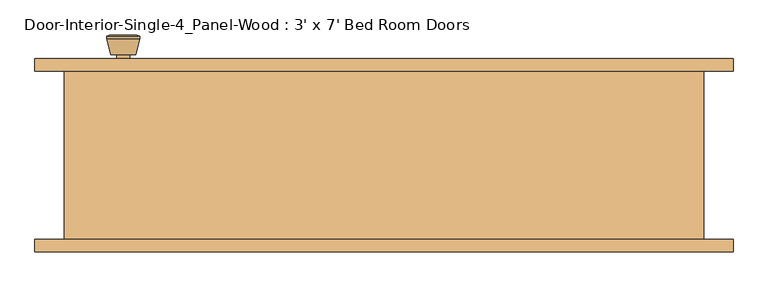
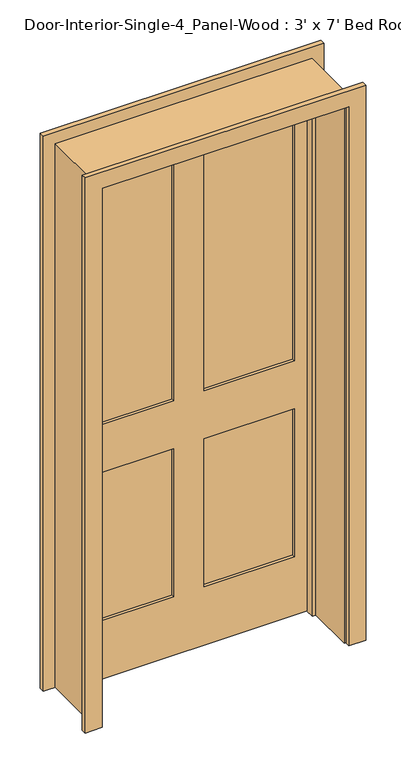
"""IFC4 building model written with IfcOpenShell, lengths in millimetres: door geometry, Door-Interior-Single-4_Panel-Wood : 3' x 7' Bed Room Doors."""

from ifc_helpers import new_model, si_unit, point, frame, frame_2d, origin, place, context, project, spatial, polyline, circle_curve, trimmed, segment, composite_curve, outline, extrude, faceted_brep, source, transform, mapped, element, save
from ifc_brep_helpers import plane_surface, cylinder_surface, revolved_surface, advanced_brep


def door_interior_single_4_panel_wood_3_x_7_bed_room_doors_330f8e7c(model_context):
    return source(origin(), model_context, "Body", "SolidModel", [
        advanced_brep(
        [(-393.7, 82.9, 914.4), (-383.7, 82.9, 914.4), (-403.7, 82.9, 914.4), (-373.2241324, 33.9, 914.4), (-393.7, 33.9, 914.4), (-414.1758676, 33.9, 914.4), (-368.7, 35.7278681, 914.4), (-418.7, 35.7278681, 914.4), (-368.7, 39.1915463, 914.4), (-418.7, 39.1915463, 914.4), (-375.063764, 63.9, 914.4), (-412.336236, 63.9, 914.4), (-383.7, 63.9, 914.4), (-403.7, 63.9, 914.4)],
        [
            (0, 1),
            (1, 2, circle_curve(frame((-393.7, 82.9, 914.4), z_axis=(0.0, 1.0, 0.0), x_axis=(-1.0, 0.0, 0.0)), 10.0)),
            (2, 0),
            (2, 1, circle_curve(frame((-393.7, 82.9, 914.4), z_axis=(0.0, 1.0, 0.0), x_axis=(-1.0, 0.0, 0.0)), 10.0)),
            (3, 4),
            (4, 5),
            (5, 3, circle_curve(frame((-393.7, 33.9, 914.4), z_axis=(0.0, -1.0, 0.0), x_axis=(-1.0, 0.0, 0.0)), 20.4758676)),
            (3, 5, circle_curve(frame((-393.7, 33.9, 914.4), z_axis=(0.0, -1.0, 0.0), x_axis=(-1.0, 0.0, 0.0)), 20.4758676)),
            (6, 3),
            (5, 7),
            (7, 6, circle_curve(frame((-393.7, 35.7278681, 914.4), z_axis=(0.0, -1.0, 0.0), x_axis=(-1.0, 0.0, 0.0)), 25.0)),
            (6, 7, circle_curve(frame((-393.7, 35.7278681, 914.4), z_axis=(0.0, -1.0, 0.0), x_axis=(-1.0, 0.0, 0.0)), 25.0)),
            (8, 6),
            (7, 9),
            (9, 8, circle_curve(frame((-393.7, 39.1915463, 914.4), z_axis=(0.0, -1.0, 0.0), x_axis=(-1.0, 0.0, 0.0)), 25.0)),
            (8, 9, circle_curve(frame((-393.7, 39.1915463, 914.4), z_axis=(0.0, -1.0, 0.0), x_axis=(-1.0, 0.0, 0.0)), 25.0)),
            (10, 8),
            (9, 11),
            (11, 10, circle_curve(frame((-393.7, 63.9, 914.4), z_axis=(0.0, -1.0, 0.0), x_axis=(-1.0, 0.0, 0.0)), 18.636236)),
            (10, 11, circle_curve(frame((-393.7, 63.9, 914.4), z_axis=(0.0, -1.0, 0.0), x_axis=(-1.0, 0.0, 0.0)), 18.636236)),
            (12, 10),
            (11, 13),
            (13, 12, circle_curve(frame((-393.7, 63.9, 914.4), z_axis=(0.0, -1.0, 0.0), x_axis=(-1.0, 0.0, 0.0)), 10.0)),
            (12, 13, circle_curve(frame((-393.7, 63.9, 914.4), z_axis=(0.0, -1.0, 0.0), x_axis=(-1.0, 0.0, 0.0)), 10.0)),
            (1, 12),
            (13, 2),
        ],
        [
            plane_surface(frame((-393.7, 82.9, 914.4), z_axis=(0.0, 1.0, 0.0), x_axis=(-1.0, 0.0, 0.0))),
            plane_surface(frame((-393.7, 33.9, 914.4), z_axis=(0.0, -1.0, 0.0), x_axis=(-1.0, 0.0, 0.0))),
            revolved_surface(polyline([(-414.1758676, 33.9, 914.4), (-418.7, 35.7278681, 914.4)]), (-393.7, 82.9, 914.4), (0.0, 1.0, 0.0)),
            cylinder_surface(frame((-393.7, 82.9, 914.4), z_axis=(0.0, 1.0, 0.0), x_axis=(-1.0, 0.0, 0.0)), 25.0),
            revolved_surface(polyline([(-418.7, 39.1915463, 914.4), (-412.336236, 63.9, 914.4)]), (-393.7, 82.9, 914.4), (0.0, 1.0, 0.0)),
            plane_surface(frame((-393.7, 63.9, 914.4), z_axis=(0.0, 1.0, 0.0), x_axis=(-1.0, 0.0, 0.0))),
            cylinder_surface(frame((-393.7, 82.9, 914.4), z_axis=(0.0, 1.0, 0.0), x_axis=(-1.0, 0.0, 0.0)), 10.0),
        ],
        [
            (0, [[1, 2, 3]]),
            (0, [[-3, 4, -1]]),
            (1, [[5, 6, 7]]),
            (1, [[-6, -5, 8]]),
            (2, [[9, -7, 10, 11]]),
            (2, [[-10, -8, -9, 12]]),
            (3, [[13, -11, 14, 15]]),
            (3, [[-14, -12, -13, 16]]),
            (4, [[17, -15, 18, 19]]),
            (4, [[-18, -16, -17, 20]]),
            (5, [[21, -19, 22, 23]]),
            (5, [[-22, -20, -21, 24]]),
            (6, [[25, -23, 26, -2]]),
            (6, [[-26, -24, -25, -4]]),
        ],
    ),
        extrude(outline(composite_curve([segment(trimmed(circle_curve(frame_2d((914.4, -393.7)), 30.0), [point((914.4, -423.7))], [point((914.4, -363.7))], False, "CARTESIAN"), True, "CONTINUOUS"), segment(trimmed(circle_curve(frame_2d((914.4, -393.7)), 30.0), [point((914.4, -363.7))], [point((914.4, -423.7))], False, "CARTESIAN"), True, "CONTINUOUS")], self_intersect=False)), frame((0.0, 82.9, 0.0), z_axis=(0.0, 1.0, 0.0), x_axis=(0.0, 0.0, 1.0)), (0.0, 0.0, 1.0), 6.0),
        advanced_brep(
        [(-393.7, 129.825, 914.4), (-403.7, 129.825, 914.4), (-383.7, 129.825, 914.4), (-373.2241324, 178.825, 914.4), (-414.1758676, 178.825, 914.4), (-393.7, 178.825, 914.4), (-368.7, 176.9971319, 914.4), (-418.7, 176.9971319, 914.4), (-368.7, 173.5334537, 914.4), (-418.7, 173.5334537, 914.4), (-375.063764, 148.825, 914.4), (-412.336236, 148.825, 914.4), (-383.7, 148.825, 914.4), (-403.7, 148.825, 914.4)],
        [
            (0, 1),
            (1, 2, circle_curve(frame((-393.7, 129.825, 914.4), z_axis=(0.0, -1.0, 0.0), x_axis=(-1.0, 0.0, 0.0)), 10.0)),
            (2, 0),
            (2, 1, circle_curve(frame((-393.7, 129.825, 914.4), z_axis=(0.0, -1.0, 0.0), x_axis=(-1.0, 0.0, 0.0)), 10.0)),
            (3, 4, circle_curve(frame((-393.7, 178.825, 914.4), z_axis=(0.0, 1.0, 0.0), x_axis=(-1.0, 0.0, 0.0)), 20.4758676)),
            (4, 5),
            (5, 3),
            (4, 3, circle_curve(frame((-393.7, 178.825, 914.4), z_axis=(0.0, 1.0, 0.0), x_axis=(-1.0, 0.0, 0.0)), 20.4758676)),
            (6, 7, circle_curve(frame((-393.7, 176.9971319, 914.4), z_axis=(0.0, 1.0, 0.0), x_axis=(-1.0, 0.0, 0.0)), 25.0)),
            (7, 4),
            (3, 6),
            (7, 6, circle_curve(frame((-393.7, 176.9971319, 914.4), z_axis=(0.0, 1.0, 0.0), x_axis=(-1.0, 0.0, 0.0)), 25.0)),
            (8, 9, circle_curve(frame((-393.7, 173.5334537, 914.4), z_axis=(0.0, 1.0, 0.0), x_axis=(-1.0, 0.0, 0.0)), 25.0)),
            (9, 7),
            (6, 8),
            (9, 8, circle_curve(frame((-393.7, 173.5334537, 914.4), z_axis=(0.0, 1.0, 0.0), x_axis=(-1.0, 0.0, 0.0)), 25.0)),
            (10, 11, circle_curve(frame((-393.7, 148.825, 914.4), z_axis=(0.0, 1.0, 0.0), x_axis=(-1.0, 0.0, 0.0)), 18.636236)),
            (11, 9),
            (8, 10),
            (11, 10, circle_curve(frame((-393.7, 148.825, 914.4), z_axis=(0.0, 1.0, 0.0), x_axis=(-1.0, 0.0, 0.0)), 18.636236)),
            (12, 13, circle_curve(frame((-393.7, 148.825, 914.4), z_axis=(0.0, 1.0, 0.0), x_axis=(-1.0, 0.0, 0.0)), 10.0)),
            (13, 11),
            (10, 12),
            (13, 12, circle_curve(frame((-393.7, 148.825, 914.4), z_axis=(0.0, 1.0, 0.0), x_axis=(-1.0, 0.0, 0.0)), 10.0)),
            (1, 13),
            (12, 2),
        ],
        [
            plane_surface(frame((-393.7, 129.825, 914.4), z_axis=(0.0, -1.0, 0.0), x_axis=(-1.0, 0.0, 0.0))),
            plane_surface(frame((-393.7, 178.825, 914.4), z_axis=(0.0, 1.0, 0.0), x_axis=(-1.0, 0.0, 0.0))),
            revolved_surface(polyline([(-414.1758676, 178.825, 914.4), (-418.7, 176.9971319, 914.4)]), (-393.7, 129.825, 914.4), (0.0, -1.0, 0.0)),
            cylinder_surface(frame((-393.7, 129.825, 914.4), z_axis=(0.0, -1.0, 0.0), x_axis=(-1.0, 0.0, 0.0)), 25.0),
            revolved_surface(polyline([(-418.7, 173.5334537, 914.4), (-412.336236, 148.825, 914.4)]), (-393.7, 129.825, 914.4), (0.0, -1.0, 0.0)),
            plane_surface(frame((-393.7, 148.825, 914.4), z_axis=(0.0, -1.0, 0.0), x_axis=(-1.0, 0.0, 0.0))),
            cylinder_surface(frame((-393.7, 129.825, 914.4), z_axis=(0.0, -1.0, 0.0), x_axis=(-1.0, 0.0, 0.0)), 10.0),
        ],
        [
            (0, [[1, 2, 3]]),
            (0, [[-3, 4, -1]]),
            (1, [[5, 6, 7]]),
            (1, [[8, -7, -6]]),
            (2, [[9, 10, -5, 11]]),
            (2, [[12, -11, -8, -10]]),
            (3, [[13, 14, -9, 15]]),
            (3, [[16, -15, -12, -14]]),
            (4, [[17, 18, -13, 19]]),
            (4, [[20, -19, -16, -18]]),
            (5, [[21, 22, -17, 23]]),
            (5, [[24, -23, -20, -22]]),
            (6, [[-2, 25, -21, 26]]),
            (6, [[-4, -26, -24, -25]]),
        ],
    ),
        extrude(outline(composite_curve([segment(trimmed(circle_curve(frame_2d((914.4, -393.7)), 30.0), [point((914.4, -423.7))], [point((914.4, -363.7))], False, "CARTESIAN"), True, "CONTINUOUS"), segment(trimmed(circle_curve(frame_2d((914.4, -393.7)), 30.0), [point((914.4, -363.7))], [point((914.4, -423.7))], False, "CARTESIAN"), True, "CONTINUOUS")], self_intersect=False)), frame((0.0, 123.825, 0.0), z_axis=(0.0, 1.0, 0.0), x_axis=(0.0, 0.0, 1.0)), (0.0, 0.0, 1.0), 6.0),
        faceted_brep([(482.6, 123.825, 0.0), (482.6, -130.175, 0.0), (457.2, -130.175, 0.0), (457.2, 53.975, 0.0), (444.5, 53.975, 0.0), (444.5, 88.9, 0.0), (457.2, 88.9, 0.0), (457.2, 123.825, 0.0), (482.6, 123.825, 2159.0), (482.6, -130.175, 2159.0), (-482.6, -130.175, 2159.0), (-482.6, -130.175, 0.0), (-457.2, -130.175, 0.0), (-457.2, -130.175, 2133.6), (457.2, -130.175, 2133.6), (457.2, 53.975, 2133.6), (-457.2, 53.975, 2133.6), (-457.2, 53.975, 0.0), (-444.5, 53.975, 0.0), (-444.5, 53.975, 2120.9), (444.5, 53.975, 2120.9), (444.5, 88.9, 2120.9), (-444.5, 88.9, 2120.9), (-444.5, 88.9, 0.0), (-457.2, 88.9, 0.0), (-457.2, 88.9, 2133.6), (457.2, 88.9, 2133.6), (457.2, 123.825, 2133.6), (-457.2, 123.825, 2133.6), (-457.2, 123.825, 0.0), (-482.6, 123.825, 0.0), (-482.6, 123.825, 2159.0)], [[[0, 1, 2, 3, 4, 5, 6, 7]], [[1, 0, 8, 9]], [[2, 1, 9, 10, 11, 12, 13, 14]], [[3, 2, 14, 15]], [[4, 3, 15, 16, 17, 18, 19, 20]], [[5, 4, 20, 21]], [[6, 5, 21, 22, 23, 24, 25, 26]], [[7, 6, 26, 27]], [[0, 7, 27, 28, 29, 30, 31, 8]], [[9, 8, 31, 10]], [[15, 14, 13, 16]], [[21, 20, 19, 22]], [[27, 26, 25, 28]], [[30, 29, 24, 23, 18, 17, 12, 11]], [[10, 31, 30, 11]], [[16, 13, 12, 17]], [[22, 19, 18, 23]], [[28, 25, 24, 29]]]),
        extrude(outline(polyline([(2133.6, -457.2), (0.0, -457.2), (0.0, 457.2), (2133.6, 457.2), (2133.6, -457.2)]), holes=[polyline([(2014.5375, 57.15), (2014.5375, 396.875), (1009.65, 396.875), (1009.65, 57.15), (2014.5375, 57.15)]), polyline([(1009.65, -57.15), (1009.65, -396.875), (2014.5375, -396.875), (2014.5375, -57.15), (1009.65, -57.15)]), polyline([(819.15, 57.15), (819.15, 396.875), (231.775, 396.875), (231.775, 57.15), (819.15, 57.15)]), polyline([(231.775, -57.15), (231.775, -396.875), (819.15, -396.875), (819.15, -57.15), (231.775, -57.15)])]), frame((0.0, 88.9, 0.0), z_axis=(0.0, 1.0, 0.0), x_axis=(0.0, 0.0, 1.0)), (0.0, 0.0, 1.0), 34.925),
        extrude(outline(polyline([(396.875, 100.5416667), (57.15, 100.5416667), (57.15, 112.1833333), (396.875, 112.1833333), (396.875, 100.5416667)])), frame((0.0, 0.0, 1009.65), z_axis=(0.0, 0.0, 1.0), x_axis=(1.0, 0.0, 0.0)), (0.0, 0.0, 1.0), 1004.8875),
        extrude(outline(polyline([(-57.15, 100.5416667), (-396.875, 100.5416667), (-396.875, 112.1833333), (-57.15, 112.1833333), (-57.15, 100.5416667)])), frame((0.0, 0.0, 1009.65), z_axis=(0.0, 0.0, 1.0), x_axis=(1.0, 0.0, 0.0)), (0.0, 0.0, 1.0), 1004.8875),
        extrude(outline(polyline([(396.875, 100.5416667), (57.15, 100.5416667), (57.15, 112.1833333), (396.875, 112.1833333), (396.875, 100.5416667)])), frame((0.0, 0.0, 231.775), z_axis=(0.0, 0.0, 1.0), x_axis=(1.0, 0.0, 0.0)), (0.0, 0.0, 1.0), 587.375),
        extrude(outline(polyline([(-57.15, 100.5416667), (-396.875, 100.5416667), (-396.875, 112.1833333), (-57.15, 112.1833333), (-57.15, 100.5416667)])), frame((0.0, 0.0, 231.775), z_axis=(0.0, 0.0, 1.0), x_axis=(1.0, 0.0, 0.0)), (0.0, 0.0, 1.0), 587.375),
        extrude(outline(polyline([(0.0, 463.55), (0.0, 527.05), (2203.45, 527.05), (2203.45, -527.05), (0.0, -527.05), (0.0, -463.55), (2139.95, -463.55), (2139.95, 463.55), (0.0, 463.55)])), frame((0.0, 123.825, 0.0), z_axis=(0.0, 1.0, 0.0), x_axis=(0.0, 0.0, 1.0)), (0.0, 0.0, 1.0), 19.05),
        extrude(outline(polyline([(0.0, 463.55), (0.0, 527.05), (2203.45, 527.05), (2203.45, -527.05), (0.0, -527.05), (0.0, -463.55), (2139.95, -463.55), (2139.95, 463.55), (0.0, 463.55)])), frame((0.0, -149.225, 0.0), z_axis=(0.0, 1.0, 0.0), x_axis=(0.0, 0.0, 1.0)), (0.0, 0.0, 1.0), 19.05),
    ])


if __name__ == "__main__":
    model = new_model("IFC4")
    model_context = context("Model", 3, world=origin())
    ifc_project = project(units=[si_unit("LENGTHUNIT", "METRE", prefix="MILLI")], contexts=[model_context])
    site = spatial("IfcSite", under=ifc_project)
    building = spatial("IfcBuilding", under=site)
    placement = place(None, origin())
    door_interior_single_4_panel_wood_3_x_7_bed_room_doors_shape = door_interior_single_4_panel_wood_3_x_7_bed_room_doors_330f8e7c(model_context)
    element("IfcDoor", 1, ObjectType="Door-Interior-Single-4_Panel-Wood : 3' x 7' Bed Room Doors", at=placement, inside=building, context=model_context, shape_type="MappedRepresentation", body=[
        mapped(door_interior_single_4_panel_wood_3_x_7_bed_room_doors_shape, transform((0.0, 0.0, 0.0), x_axis=(1.0, 0.0, 0.0), y_axis=(0.0, 1.0, 0.0), z_axis=(0.0, 0.0, 1.0))),
    ])
    save(model, "model.ifc")

# Revit data of these elements
# Type "Door-Interior-Single-4_Panel-Wood : 3' x 7' Bed Room Doors"
#   Type Mark = "13"
#   Assembly Code = "C1020300"
#   Analytic Construction = "Wooden"
#   Top Rail = 0' - 4 11/16"
#   Thickness = 0' - 1 3/8"
#   Thermal Resistance (R) = 2.5876 (h·ft²·°F)/BTU
#   Swing Angle [instance default] = 90.00°
#   Stiles = 0' - 2 3/8"
#   Rough Width = 3' - 2"
#   Rough Height = 7' - 1"
#   Mullion = 0' - 4 1/2"
#   Lock Rail = 0' - 7 1/2"
#   Height = 7' - 0"
#   Width = 3' - 0"
#   Heat Transfer Coefficient (U) = 0.3865 BTU/(h·ft²·°F)
#   Bottom Rail = 0' - 9 1/8"
#   Trim Material = Cherry
#   Panel Material = Cherry
#   Frame Material = Cherry
#   Door Handle Material = Aluminum
#   Visual Light Transmittance = 0
#   Solar Heat Gain Coefficient = 0
#   Wall Closure = (empty or 0)
#   Function = (empty or 0)
# Element 1 (IfcDoor, "Door-Interior-Single-4_Panel-Wood : 3' x 7' Bed Room Doors")
#   Materials on its faces: "Cherry", "Aluminum"
# Materials
#   "Cherry": class "Wood", colour RGB 226 177 128, transparency 0, Description = "Prunus Serotina", Cost = 0
#   "Aluminum": class "Metal", colour RGB 247 247 247, transparency 0, Description = "Aluminum 6061", Cost = 0
